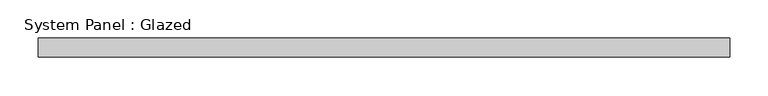
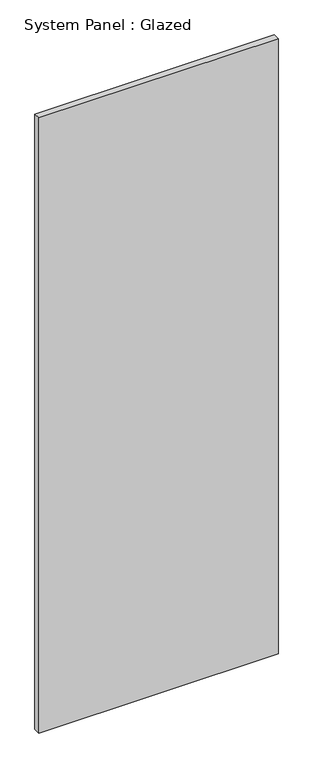
"""IFC4 building model written with IfcOpenShell, lengths in millimetres: plate geometry, System Panel : Glazed."""

from ifc_helpers import new_model, si_unit, origin, origin_with_axes, place, context, project, spatial, polyline, outline, extrude, source, transform, mapped, element, save


def system_panel_glazed_39fbb70d(model_context):
    return source(origin(), model_context, "Body", "SweptSolid", [
        extrude(outline(polyline([(451.25, 24.5), (-451.25, 24.5), (-451.25, 49.5), (451.25, 49.5), (451.25, 24.5)])), origin_with_axes(), (0.0, 0.0, 1.0), 2452.5),
    ])


if __name__ == "__main__":
    model = new_model("IFC4")
    model_context = context("Model", 3, world=origin())
    ifc_project = project(units=[si_unit("LENGTHUNIT", "METRE", prefix="MILLI")], contexts=[model_context])
    site = spatial("IfcSite", under=ifc_project)
    building = spatial("IfcBuilding", under=site)
    placement = place(None, origin())
    system_panel_glazed_shape = system_panel_glazed_39fbb70d(model_context)
    element("IfcPlate", 1, ObjectType="System Panel : Glazed", at=placement, inside=building, context=model_context, shape_type="MappedRepresentation", body=[
        mapped(system_panel_glazed_shape, transform((0.0, 0.0, 0.0), x_axis=(1.0, 0.0, 0.0), y_axis=(0.0, 1.0, 0.0), z_axis=(0.0, 0.0, 1.0))),
    ])
    save(model, "model.ifc")

# Revit data of these elements
# Type "System Panel : Glazed"
#   Construction Type Id = "GSP4R"
#   Analytic Construction = "1/8 in Pilkington single glazing"
#   Visual Light Transmittance = 0.9
#   Solar Heat Gain Coefficient = 0.86
#   Heat Transfer Coefficient (U) = 6.7069 W/(m²·K)
#   Define Thermal Properties by = 1
# Element 1 (IfcPlate, "System Panel : Glazed")
#   Materials on its faces: "Glass"
# Materials
#   "Glass": class "Glass", colour RGB 245 245 243, transparency 1, Description = "Soda Lime Glass", Cost = 0
